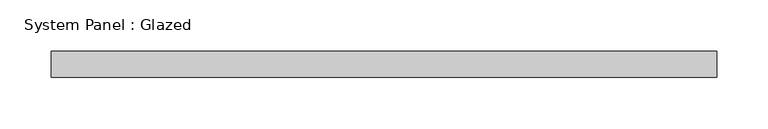
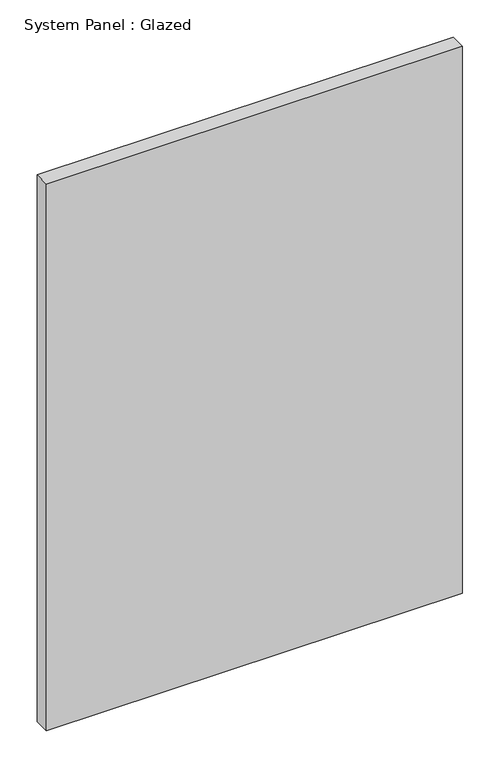
"""IFC4 building model written with IfcOpenShell, lengths in millimetres: plate geometry, System Panel : Glazed."""

from ifc_helpers import new_model, si_unit, origin, origin_with_axes, place, context, project, spatial, polyline, outline, extrude, source, transform, mapped, element, save


def system_panel_glazed_a28047ed(model_context):
    return source(origin(), model_context, "Body", "SweptSolid", [
        extrude(outline(polyline([(323.85, 19.05), (-323.85, 19.05), (-323.85, 44.45), (323.85, 44.45), (323.85, 19.05)])), origin_with_axes(), (0.0, 0.0, 1.0), 900.0180153),
    ])


if __name__ == "__main__":
    model = new_model("IFC4")
    model_context = context("Model", 3, world=origin())
    ifc_project = project(units=[si_unit("LENGTHUNIT", "METRE", prefix="MILLI")], contexts=[model_context])
    site = spatial("IfcSite", under=ifc_project)
    building = spatial("IfcBuilding", under=site)
    placement = place(None, origin())
    system_panel_glazed_shape = system_panel_glazed_a28047ed(model_context)
    element("IfcPlate", 1, ObjectType="System Panel : Glazed", at=placement, inside=building, context=model_context, shape_type="MappedRepresentation", body=[
        mapped(system_panel_glazed_shape, transform((0.0, 0.0, 0.0), x_axis=(1.0, 0.0, 0.0), y_axis=(0.0, 1.0, 0.0), z_axis=(0.0, 0.0, 1.0))),
    ])
    save(model, "model.ifc")

# Revit data of these elements
# Type "System Panel : Glazed"
#   Construction Type Id = "GSP4R"
#   Analytic Construction = "1/8 in Pilkington single glazing"
#   Visual Light Transmittance = 0.9
#   Solar Heat Gain Coefficient = 0.86
#   Heat Transfer Coefficient (U) = 1.18115 BTU/(h·ft²·°F)
#   Define Thermal Properties by = 1
# Element 1 (IfcPlate, "System Panel : Glazed")
#   Materials on its faces: "Glass"
# Materials
#   "Glass": class "Glass", colour RGB 0 128 192, transparency 0.75, Description = "Soda Lime Glass", Cost = 0
